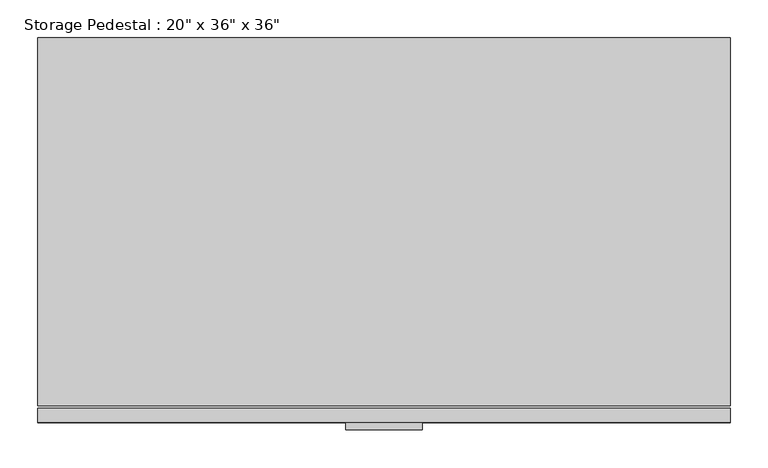
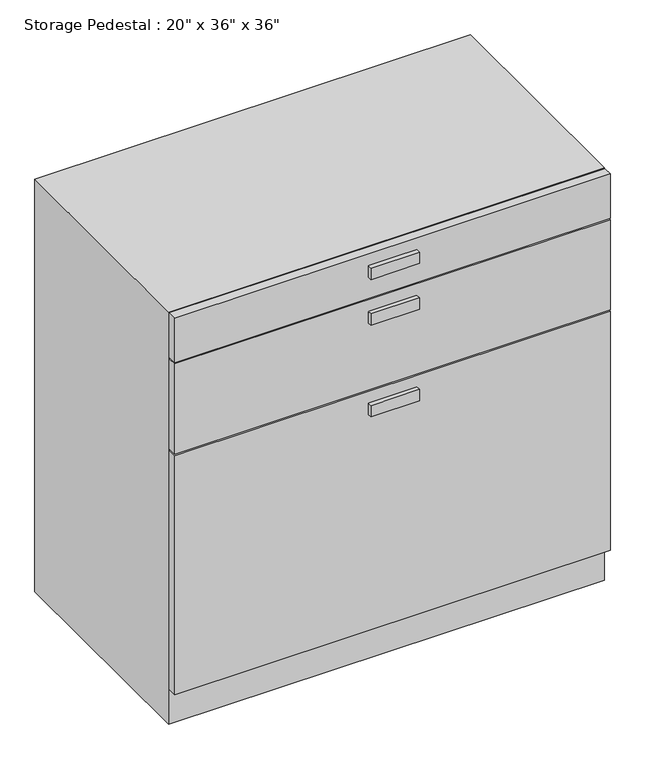
"""IFC4 building model written with IfcOpenShell, lengths in millimetres: furniture geometry."""

from ifc_helpers import new_model, si_unit, frame, origin, origin_with_axes, place, context, project, spatial, polyline, outline, extrude, source, transform, mapped, element, save


def furniture_e1dba61b(model_context):
    return source(origin(), model_context, "Body", "SweptSolid", [
        extrude(outline(polyline([(277.1774861, -1188.3183761), (-637.2225139, -1188.3183761), (-637.2225139, -1169.2683761), (277.1774861, -1169.2683761), (277.1774861, -1188.3183761)])), frame((0.0, 0.0, 79.375), z_axis=(0.0, 0.0, 1.0), x_axis=(1.0, 0.0, 0.0)), (0.0, 0.0, 1.0), 530.225),
        extrude(outline(polyline([(277.1774861, -1188.3183761), (-637.2225139, -1188.3183761), (-637.2225139, -1169.2683761), (277.1774861, -1169.2683761), (277.1774861, -1188.3183761)])), frame((0.0, 0.0, 612.775), z_axis=(0.0, 0.0, 1.0), x_axis=(1.0, 0.0, 0.0)), (0.0, 0.0, 1.0), 200.025),
        extrude(outline(polyline([(277.1774861, -1188.3183761), (-637.2225139, -1188.3183761), (-637.2225139, -1169.2683761), (277.1774861, -1169.2683761), (277.1774861, -1188.3183761)])), frame((0.0, 0.0, 815.975), z_axis=(0.0, 0.0, 1.0), x_axis=(1.0, 0.0, 0.0)), (0.0, 0.0, 1.0), 98.425),
        extrude(outline(polyline([(277.1774861, -680.3183761), (277.1774861, -1166.0933761), (-637.2225139, -1166.0933761), (-637.2225139, -680.3183761), (277.1774861, -680.3183761)])), origin_with_axes(), (0.0, 0.0, 1.0), 914.4),
        extrude(outline(polyline([(-129.2225139, -1197.8433761), (-230.8225139, -1197.8433761), (-230.8225139, -1188.3183761), (-129.2225139, -1188.3183761), (-129.2225139, -1197.8433761)])), frame((0.0, 0.0, 863.6), z_axis=(0.0, 0.0, 1.0), x_axis=(1.0, 0.0, 0.0)), (0.0, 0.0, 1.0), 25.4),
        extrude(outline(polyline([(-129.2225139, -1197.8433761), (-230.8225139, -1197.8433761), (-230.8225139, -1188.3183761), (-129.2225139, -1188.3183761), (-129.2225139, -1197.8433761)])), frame((0.0, 0.0, 762.0), z_axis=(0.0, 0.0, 1.0), x_axis=(1.0, 0.0, 0.0)), (0.0, 0.0, 1.0), 25.4),
        extrude(outline(polyline([(-129.2225139, -1197.8433761), (-230.8225139, -1197.8433761), (-230.8225139, -1188.3183761), (-129.2225139, -1188.3183761), (-129.2225139, -1197.8433761)])), frame((0.0, 0.0, 558.8), z_axis=(0.0, 0.0, 1.0), x_axis=(1.0, 0.0, 0.0)), (0.0, 0.0, 1.0), 25.4),
    ])


if __name__ == "__main__":
    model = new_model("IFC4")
    model_context = context("Model", 3, world=origin())
    ifc_project = project(units=[si_unit("LENGTHUNIT", "METRE", prefix="MILLI")], contexts=[model_context])
    site = spatial("IfcSite", under=ifc_project)
    building = spatial("IfcBuilding", under=site)
    placement = place(None, origin())
    furniture_shape = furniture_e1dba61b(model_context)
    element("IfcFurniture", 1, ObjectType="Storage Pedestal : 20\" x 36\" x 36\"", at=placement, inside=building, context=model_context, shape_type="MappedRepresentation", body=[
        mapped(furniture_shape, transform((0.0, 0.0, 0.0), x_axis=(1.0, 0.0, 0.0), y_axis=(0.0, 1.0, 0.0), z_axis=(0.0, 0.0, 1.0))),
    ])
    save(model, "model.ifc")

# Revit data of these elements
# Type "Storage Pedestal : 20\" x 36\" x 36\""
#   Assembly Code = "E2020"
#   Depth = 1' - 8"
#   Height = 3' - 0"
#   Width = 3' - 0"
#   Cabinet Material = Steel, Paint Finish, Ivory, Glossy
#   Handles Material = Steel, Chrome Plated
#   Default Elevation = 0
# Element 1 (IfcFurniture, "Storage Pedestal : 20\" x 36\" x 36\"")
#   Materials on its faces: "Steel, Paint Finish, Ivory, Glossy", "Steel, Chrome Plated"
# Materials
#   "Steel, Paint Finish, Ivory, Glossy": class "Metal", colour RGB 247 247 239, transparency 0, Description = "Steel, paint finish, ivory, glossy", Cost = 0
#   "Steel, Chrome Plated": class "Metal", colour RGB 17 17 17, transparency 0, Description = "Chromiuim plated steel", Cost = 0
